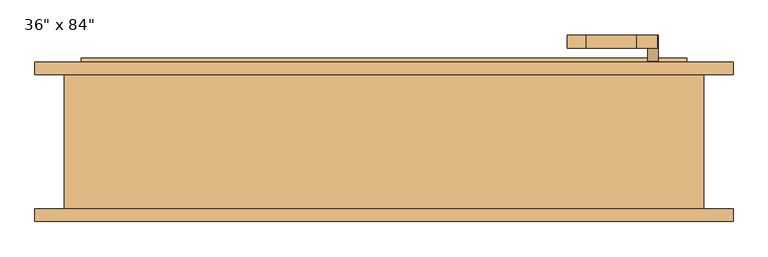
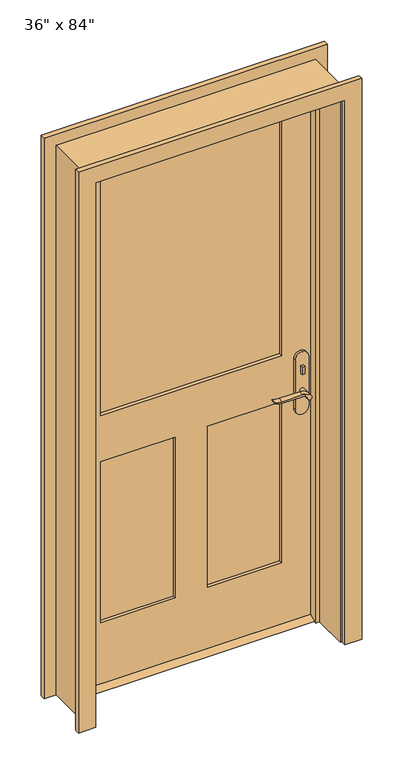
"""IFC4 building model written with IfcOpenShell, lengths in millimetres: door geometry."""

from ifc_helpers import new_model, si_unit, point, frame, frame_2d, origin, place, context, project, spatial, polyline, circle_curve, trimmed, segment, composite_curve, outline, extrude, faceted_brep, source, transform, mapped, element, save


def door_3d09584f(model_context):
    return source(origin(), model_context, "Body", "SolidModel", [
        extrude(outline(polyline([(63.5, 12.7), (98.425, 12.7), (123.825, 0.0), (38.1, 0.0), (63.5, 12.7)])), frame((-457.2, 0.0, 0.0), z_axis=(1.0, 0.0, 0.0), x_axis=(0.0, 1.0, 0.0)), (0.0, 0.0, 1.0), 914.4),
        extrude(outline(polyline([(411.4, 43.5), (401.4, 43.5), (401.4, 53.5), (411.4, 53.5), (411.4, 43.5)])), frame((0.0, 0.0, 981.9), z_axis=(0.0, 0.0, 1.0), x_axis=(1.0, 0.0, 0.0)), (0.0, 0.0, 1.0), 30.0),
        extrude(outline(composite_curve([segment(trimmed(circle_curve(frame_2d((996.9, 406.4)), 8.0), [point((996.9, 398.4))], [point((996.9, 414.4))], False, "CARTESIAN"), True, "CONTINUOUS"), segment(trimmed(circle_curve(frame_2d((996.9, 406.4)), 8.0), [point((996.9, 414.4))], [point((996.9, 398.4))], False, "CARTESIAN"), True, "CONTINUOUS")], self_intersect=False)), frame((0.0, 108.425, 0.0), z_axis=(0.0, 1.0, 0.0), x_axis=(0.0, 0.0, 1.0)), (0.0, 0.0, 1.0), 10.0),
        extrude(outline(composite_curve([segment(trimmed(circle_curve(frame_2d((897.1555521, 382.7324871)), 37.2832219), [point((919.0523287, 412.9081363))], [point((934.4, 381.0325667))], False, "CARTESIAN"), True, "CONTINUOUS"), segment(polyline([(934.4, 381.0325667), (934.4, 304.7564091)]), True, "CONTINUOUS"), segment(trimmed(circle_curve(frame_2d((1017.6850638, 304.8227909)), 83.2850902), [point((934.4, 304.7564091))], [point((939.4, 276.4))], True, "CARTESIAN"), True, "CONTINUOUS"), segment(polyline([(939.4, 276.4), (936.6135558, 276.4)]), True, "CONTINUOUS"), segment(trimmed(circle_curve(frame_2d((986.6709207, 308.3396612)), 59.3791355), [point((936.6135558, 276.4))], [point((927.4, 304.7564091))], False, "CARTESIAN"), True, "CONTINUOUS"), segment(polyline([(927.4, 304.7564091), (927.4, 381.0138099)]), True, "CONTINUOUS"), segment(trimmed(circle_curve(frame_2d((909.2738613, 381.0138099)), 18.1261387), [point((927.4, 381.0138099))], [point((914.4, 398.4))], True, "CARTESIAN"), True, "CONTINUOUS"), segment(trimmed(circle_curve(frame_2d((914.4, 406.4)), 8.0), [point((914.4, 398.4))], [point((919.0523287, 412.9081363))], False, "CARTESIAN"), True, "CONTINUOUS")], self_intersect=False)), frame((0.0, 3.5, 0.0), z_axis=(0.0, 1.0, 0.0), x_axis=(0.0, 0.0, 1.0)), (0.0, 0.0, 1.0), 20.0),
        extrude(outline(composite_curve([segment(trimmed(circle_curve(frame_2d((914.4, 406.4)), 8.0), [point((914.3999903, 398.4))], [point((919.0523287, 412.9081363))], False, "CARTESIAN"), True, "CONTINUOUS"), segment(trimmed(circle_curve(frame_2d((897.1555521, 382.7324871)), 37.2832219), [point((919.0523287, 412.9081363))], [point((934.4, 381.0325667))], False, "CARTESIAN"), True, "CONTINUOUS"), segment(polyline([(934.4, 381.0325667), (934.4, 304.7564091)]), True, "CONTINUOUS"), segment(trimmed(circle_curve(frame_2d((1017.6850638, 304.8227909)), 83.2850902), [point((934.4, 304.7564091))], [point((939.4, 276.4))], True, "CARTESIAN"), True, "CONTINUOUS"), segment(polyline([(939.4, 276.4), (936.6135558, 276.4)]), True, "CONTINUOUS"), segment(trimmed(circle_curve(frame_2d((986.6709207, 308.3396612)), 59.3791355), [point((936.6135558, 276.4))], [point((927.4, 304.7564091))], False, "CARTESIAN"), True, "CONTINUOUS"), segment(polyline([(927.4, 304.7564091), (927.4, 381.0138122)]), True, "CONTINUOUS"), segment(trimmed(circle_curve(frame_2d((909.2738682, 381.0138122)), 18.1261318), [point((927.4, 381.0138122))], [point((914.3999903, 398.4))], True, "CARTESIAN"), True, "CONTINUOUS")], self_intersect=False)), frame((0.0, 138.425, 0.0), z_axis=(0.0, 1.0, 0.0), x_axis=(0.0, 0.0, 1.0)), (0.0, 0.0, 1.0), 20.0),
        extrude(outline(composite_curve([segment(trimmed(circle_curve(frame_2d((914.4, 406.4)), 8.0), [point((914.4, 398.4))], [point((914.4, 414.4))], False, "CARTESIAN"), True, "CONTINUOUS"), segment(trimmed(circle_curve(frame_2d((914.4, 406.4)), 8.0), [point((914.4, 414.4))], [point((914.4, 398.4))], False, "CARTESIAN"), True, "CONTINUOUS")], self_intersect=False)), frame((0.0, 23.5, 0.0), z_axis=(0.0, 1.0, 0.0), x_axis=(0.0, 0.0, 1.0)), (0.0, 0.0, 1.0), 30.0),
        extrude(outline(composite_curve([segment(trimmed(circle_curve(frame_2d((914.4, 406.4)), 8.0), [point((914.4, 398.4))], [point((914.4, 414.4))], False, "CARTESIAN"), True, "CONTINUOUS"), segment(trimmed(circle_curve(frame_2d((914.4, 406.4)), 8.0), [point((914.4, 414.4))], [point((914.4, 398.4))], False, "CARTESIAN"), True, "CONTINUOUS")], self_intersect=False)), frame((0.0, 108.425, 0.0), z_axis=(0.0, 1.0, 0.0), x_axis=(0.0, 0.0, 1.0)), (0.0, 0.0, 1.0), 30.0),
        extrude(outline(composite_curve([segment(polyline([(844.4, 431.4), (1039.4, 431.4)]), True, "CONTINUOUS"), segment(trimmed(circle_curve(frame_2d((1039.4, 406.4)), 25.0), [point((1039.4, 431.4))], [point((1039.4, 381.4))], False, "CARTESIAN"), True, "CONTINUOUS"), segment(polyline([(1039.4, 381.4), (844.4, 381.4)]), True, "CONTINUOUS"), segment(trimmed(circle_curve(frame_2d((844.4, 406.4)), 25.0), [point((844.4, 381.4))], [point((844.4, 431.4))], False, "CARTESIAN"), True, "CONTINUOUS")], self_intersect=False)), frame((0.0, 53.5, 0.0), z_axis=(0.0, 1.0, 0.0), x_axis=(0.0, 0.0, 1.0)), (0.0, 0.0, 1.0), 10.0),
        extrude(outline(composite_curve([segment(polyline([(844.4, 431.4), (1039.4, 431.4)]), True, "CONTINUOUS"), segment(trimmed(circle_curve(frame_2d((1039.4, 406.4)), 25.0), [point((1039.4, 431.4))], [point((1039.4, 381.4))], False, "CARTESIAN"), True, "CONTINUOUS"), segment(polyline([(1039.4, 381.4), (844.4, 381.4)]), True, "CONTINUOUS"), segment(trimmed(circle_curve(frame_2d((844.4, 406.4)), 25.0), [point((844.4, 381.4))], [point((844.4, 431.4))], False, "CARTESIAN"), True, "CONTINUOUS")], self_intersect=False)), frame((0.0, 98.425, 0.0), z_axis=(0.0, 1.0, 0.0), x_axis=(0.0, 0.0, 1.0)), (0.0, 0.0, 1.0), 10.0),
        extrude(outline(polyline([(2133.6, -457.2), (12.7, -457.2), (12.7, 457.2), (2133.6, 457.2), (2133.6, -457.2)]), holes=[polyline([(1066.8, -336.55), (2012.95, -336.55), (2012.95, 336.55), (1066.8, 336.55), (1066.8, -336.55)]), polyline([(885.825, -60.325), (254.0, -60.325), (254.0, -336.55), (885.825, -336.55), (885.825, -60.325)]), polyline([(885.825, 336.55), (254.0, 336.55), (254.0, 60.325), (885.825, 60.325), (885.825, 336.55)])]), frame((0.0, 63.5, 0.0), z_axis=(0.0, 1.0, 0.0), x_axis=(0.0, 0.0, 1.0)), (0.0, 0.0, 1.0), 34.925),
        faceted_brep([(482.6, 98.425, 0.0), (482.6, -104.775, 0.0), (457.2, -104.775, 0.0), (457.2, 28.575, 0.0), (444.5, 28.575, 0.0), (444.5, 63.5, 0.0), (457.2, 63.5, 0.0), (457.2, 98.425, 0.0), (482.6, 98.425, 2159.0), (482.6, -104.775, 2159.0), (-482.6, -104.775, 2159.0), (-482.6, -104.775, 0.0), (-457.2, -104.775, 0.0), (-457.2, -104.775, 2133.6), (457.2, -104.775, 2133.6), (457.2, 28.575, 2133.6), (-457.2, 28.575, 2133.6), (-457.2, 28.575, 0.0), (-444.5, 28.575, 0.0), (-444.5, 28.575, 2120.9), (444.5, 28.575, 2120.9), (444.5, 63.5, 2120.9), (-444.5, 63.5, 2120.9), (-444.5, 63.5, 0.0), (-457.2, 63.5, 0.0), (-457.2, 63.5, 2133.6), (457.2, 63.5, 2133.6), (457.2, 98.425, 2133.6), (-457.2, 98.425, 2133.6), (-457.2, 98.425, 0.0), (-482.6, 98.425, 0.0), (-482.6, 98.425, 2159.0)], [[[0, 1, 2, 3, 4, 5, 6, 7]], [[1, 0, 8, 9]], [[2, 1, 9, 10, 11, 12, 13, 14]], [[3, 2, 14, 15]], [[4, 3, 15, 16, 17, 18, 19, 20]], [[5, 4, 20, 21]], [[6, 5, 21, 22, 23, 24, 25, 26]], [[7, 6, 26, 27]], [[0, 7, 27, 28, 29, 30, 31, 8]], [[9, 8, 31, 10]], [[15, 14, 13, 16]], [[21, 20, 19, 22]], [[27, 26, 25, 28]], [[30, 29, 24, 23, 18, 17, 12, 11]], [[10, 31, 30, 11]], [[16, 13, 12, 17]], [[22, 19, 18, 23]], [[28, 25, 24, 29]]]),
        extrude(outline(polyline([(-60.325, 75.1416667), (-336.55, 75.1416667), (-336.55, 86.7833333), (-60.325, 86.7833333), (-60.325, 75.1416667)])), frame((0.0, 0.0, 254.0), z_axis=(0.0, 0.0, 1.0), x_axis=(1.0, 0.0, 0.0)), (0.0, 0.0, 1.0), 631.825),
        extrude(outline(polyline([(336.55, 75.1416667), (60.325, 75.1416667), (60.325, 86.7833333), (336.55, 86.7833333), (336.55, 75.1416667)])), frame((0.0, 0.0, 254.0), z_axis=(0.0, 0.0, 1.0), x_axis=(1.0, 0.0, 0.0)), (0.0, 0.0, 1.0), 631.825),
        extrude(outline(polyline([(336.55, 77.47), (-336.55, 77.47), (-336.55, 84.455), (336.55, 84.455), (336.55, 77.47)])), frame((0.0, 0.0, 1066.8), z_axis=(0.0, 0.0, 1.0), x_axis=(1.0, 0.0, 0.0)), (0.0, 0.0, 1.0), 946.15),
        extrude(outline(polyline([(0.0, -527.05), (0.0, -463.55), (2139.95, -463.55), (2139.95, 463.55), (0.0, 463.55), (0.0, 527.05), (2203.45, 527.05), (2203.45, -527.05), (0.0, -527.05)])), frame((0.0, -123.825, 0.0), z_axis=(0.0, 1.0, 0.0), x_axis=(0.0, 0.0, 1.0)), (0.0, 0.0, 1.0), 19.05),
        extrude(outline(polyline([(0.0, -527.05), (0.0, -463.55), (2139.95, -463.55), (2139.95, 463.55), (0.0, 463.55), (0.0, 527.05), (2203.45, 527.05), (2203.45, -527.05), (0.0, -527.05)])), frame((0.0, 98.425, 0.0), z_axis=(0.0, 1.0, 0.0), x_axis=(0.0, 0.0, 1.0)), (0.0, 0.0, 1.0), 19.05),
    ])


if __name__ == "__main__":
    model = new_model("IFC4")
    model_context = context("Model", 3, world=origin())
    ifc_project = project(units=[si_unit("LENGTHUNIT", "METRE", prefix="MILLI")], contexts=[model_context])
    site = spatial("IfcSite", under=ifc_project)
    building = spatial("IfcBuilding", under=site)
    placement = place(None, origin())
    door_shape = door_3d09584f(model_context)
    element("IfcDoor", 1, ObjectType="36\" x 84\"", at=placement, inside=building, context=model_context, shape_type="MappedRepresentation", body=[
        mapped(door_shape, transform((0.0, 0.0, 0.0), x_axis=(1.0, 0.0, 0.0), y_axis=(0.0, 1.0, 0.0), z_axis=(0.0, 0.0, 1.0))),
    ])
    save(model, "model.ifc")

# Revit data of these elements
# Type "36\" x 84\""
#   Type Mark = "11"
#   Assembly Code = "B2030100"
#   Analytic Construction = "French door, wood frame with single glass"
#   Top Rail = 0' - 4 3/4"
#   Threshold Offset [instance default] = 0' - 0 1/2"
#   Thickness = 0' - 1 3/8"
#   Thermal Resistance (R) = 1.0696 (h·ft²·°F)/BTU
#   Swing Angle [instance default] = 90.00°
#   Stiles = 0' - 4 3/4"
#   Rough Width = 3' - 2"
#   Rough Height = 7' - 1"
#   Lock Rail = 0' - 7 1/8"
#   Height = 7' - 0"
#   Width = 3' - 0"
#   Heat Transfer Coefficient (U) = 0.9350 BTU/(h·ft²·°F)
#   Door Offset [instance default] = 0' - 0"
#   Bottom Rail = 0' - 9 1/2"
#   Threshold [instance default] = yes
#   Function = 1
#   Exterior Trim [instance default] = yes
#   Trim Material = Cherry
#   Threshold Material = Cherry
#   Panel Material = Cherry
#   Glazing = Glass
#   Frame Material = Cherry
#   Door Handle Material = Aluminum
#   Visual Light Transmittance = 0
#   Solar Heat Gain Coefficient = 0
#   Wall Closure = (empty or 0)
#   Construction Type = (empty or 0)
# Element 1 (IfcDoor, "36\" x 84\"")
#   Materials on its faces: "Cherry", "Aluminum", "Glass"
# Materials
#   "Cherry": class "Wood", colour RGB 226 177 128, transparency 0, Description = "Prunus Serotina", Cost = 0
#   "Glass": class "Glass", colour RGB 0 128 192, transparency 0.75, Description = "Soda Lime Glass", Cost = 0
#   "Aluminum": class "Metal", colour RGB 247 247 247, transparency 0, Description = "Aluminum 6061", Cost = 0
